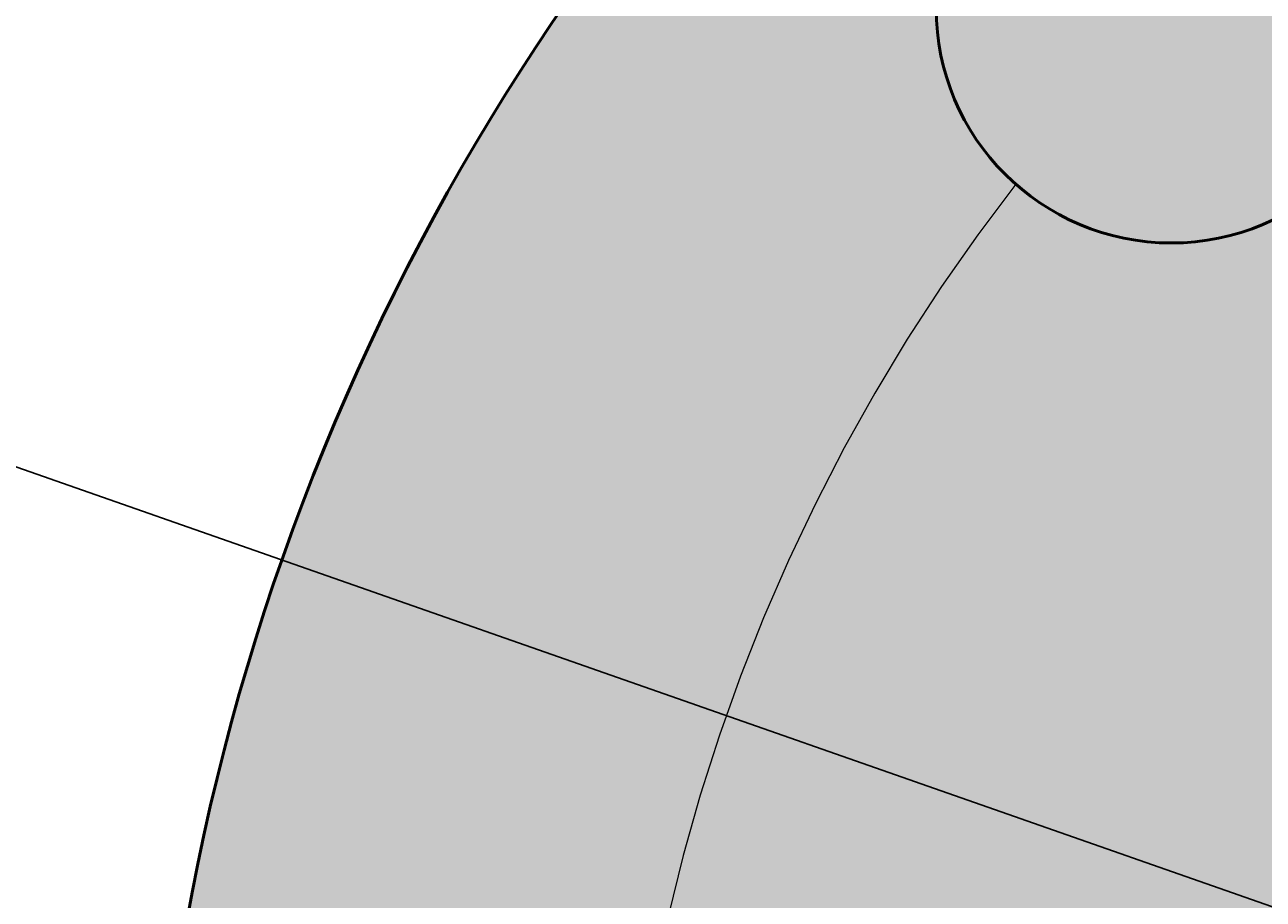
# Model space of a CAD drawing. Units: inches. Extents: x 139261 to 139415, y 52839 to 52963.
# Tile 5 of 20: x 139288 to 139314, y 52910 to 52928. Entities that reach past the tile are written whole.
import ezdxf

# ---------------------------------------------------------------- set-up
doc = ezdxf.new("R2010")
doc.units = ezdxf.units.IN
doc.header["$MEASUREMENT"] = 0
doc.linetypes.add('CENTER', pattern=[50.8, 31.75, -6.35, 6.35, -6.35])
for name, color, linetype, lineweight in [('M-CNTR', 4, 'CENTER', 18), ('M-DIMS', 2, 'Continuous', 25), ('M-HATC', 8, 'Continuous', 18), ('M-OUTL', 7, 'Continuous', 50)]:
    doc.layers.add(name, color=color, linetype=linetype, lineweight=lineweight)
doc.styles.get("Standard").update_dxf_attribs({"font": 'arial.ttf'})
doc.dimstyles.get("Standard").update_dxf_attribs({"dimtxt": 0.18, "dimasz": 0.18, "dimexe": 0.18, "dimexo": 0.0625, "dimgap": 0.09, "dimtad": 0, "dimtih": 1, "dimtoh": 1, "dimdec": 4, "dimzin": 0, "dimdsep": 46, "dimtxsty": 'Standard', "dimcen": 0.09, "dimadec": 0, "dimazin": 0, "dimtfac": 1, "dimtdec": 4, "dimtofl": 0, "dimtmove": 0, "dimatfit": 3, "dimfxl": 1, "dimtolj": 1, "dimtzin": 0, "dimarcsym": 0})

# ---------------------------------------------------------------- blocks, each defined once
blk = doc.blocks.new('*U1')
blk.add_circle((0, 0), 5)
blk = doc.blocks.new('*U2')
at = {"layer": 'M-OUTL', "color": 0, "linetype": 'ByBlock', "lineweight": -2, "transparency": 16777216, "rotation": 45.00000000000001}
blk.add_blockref('*U1', (139312.073, 52928.502), dxfattribs=at)
blk = doc.blocks.new('*D4')
at = {"layer": 'Defpoints', "color": 0, "transparency": 16777216}
for p in [(139373.053, 52923.26), (139307.661, 52877.175)]:
    blk.add_point(p, dxfattribs=at)
at = {"layer": 'M-DIMS', "color": 0, "lineweight": -2, "transparency": 16777216}
for p, q in [((139414.011, 52952.126), (139373.2, 52923.364)), ((139414.191, 52952.126), (139414.011, 52952.126)), ((139340.267, 52900.217), (139340.447, 52900.217)), ((139340.357, 52900.127), (139340.357, 52900.307))]:
    blk.add_line(p, q, dxfattribs=at)
blk.add_arc((139340.357, 52900.217), 40, 34.9168, 52.0771, dxfattribs=at)
at = {"layer": 'M-DIMS', "color": 0, "transparency": 16777216}
blk.add_solid([(139373.183, 52923.388), (139373.217, 52923.339), (139373.053, 52923.26)], dxfattribs=at)
at = {"layer": 'M-DIMS', "color": 0, "transparency": 16777216, "insert": (139414.822, 52952.126), "char_height": 0.18, "attachment_point": 5}
blk.add_mtext('\\A1;∅80.0000', dxfattribs=at)
blk = doc.blocks.new('*D5')
at = {"layer": 'Defpoints', "color": 0, "transparency": 16777216}
for p in [(139316.763, 52908.484), (139363.951, 52891.951)]:
    blk.add_point(p, dxfattribs=at)
at = {"layer": 'M-DIMS', "color": 0, "lineweight": -2, "transparency": 16777216}
for p, q in [((139262.553, 52927.414), (139262.733, 52927.414)), ((139262.733, 52927.414), (139316.593, 52908.544)), ((139340.267, 52900.217), (139340.447, 52900.217)), ((139340.357, 52900.127), (139340.357, 52900.307))]:
    blk.add_line(p, q, dxfattribs=at)
at = {"layer": 'M-DIMS', "color": 0, "transparency": 16777216}
blk.add_solid([(139316.603, 52908.572), (139316.583, 52908.515), (139316.763, 52908.484)], dxfattribs=at)
at = {"layer": 'M-DIMS', "color": 0, "transparency": 16777216, "insert": (139261.922, 52927.414), "char_height": 0.18, "attachment_point": 5}
blk.add_mtext('\\A1;∅50.0000', dxfattribs=at)
blk = doc.blocks.new('*D9')
at = {"layer": 'Defpoints', "color": 0, "transparency": 16777216}
for p in [(139302.054, 52932.357), (139378.659, 52868.078)]:
    blk.add_point(p, dxfattribs=at)
at = {"layer": 'M-DIMS', "color": 0, "lineweight": -2, "transparency": 16777216}
for p, q in [((139278.893, 52951.64), (139279.073, 52951.64)), ((139279.073, 52951.64), (139301.916, 52932.472)), ((139340.267, 52900.217), (139340.447, 52900.217)), ((139340.357, 52900.127), (139340.357, 52900.307))]:
    blk.add_line(p, q, dxfattribs=at)
at = {"layer": 'M-DIMS', "color": 0, "transparency": 16777216}
blk.add_solid([(139301.936, 52932.495), (139301.897, 52932.449), (139302.054, 52932.357)], dxfattribs=at)
at = {"layer": 'M-DIMS', "color": 0, "transparency": 16777216, "insert": (139278.506, 52951.64), "char_height": 0.18, "attachment_point": 5}
blk.add_mtext('\\A1;∅100', dxfattribs=at)

msp = doc.modelspace()

# ---------------------------------------------------------------- hatches: boundary and pattern name
at = {"layer": 'M-HATC'}
h = msp.add_hatch(color=256, dxfattribs=at)
h.dxf.hatch_style = 1
h.paths.add_polyline_path([(139290.35689, 52900.21749, 1), (139390.35689, 52900.21749, 1)])
h.paths.add_polyline_path([(139335.36666, 52939.90499, -0.01563646), (139335.35689, 52940.21749, -1), (139345.35689, 52940.21749, -0.01563646), (139345.34711, 52939.90499, -0.13461315), (139364.89157, 52931.80941, -0.691035), (139373.64116, 52928.50176, -0.21521822), (139371.94881, 52924.75216, -0.13461315), (139380.04439, 52905.20771, -0.43265224), (139385.35689, 52900.21749, -0.43265224), (139380.04439, 52895.22726, -0.13461315), (139371.94881, 52875.68281, -0.21521822), (139373.64116, 52871.93321, -0.691035), (139364.89157, 52868.62556, -0.13461315), (139345.34711, 52860.52999, -0.01563646), (139345.35689, 52860.21749, -1), (139335.35689, 52860.21749, -0.01563646), (139335.36666, 52860.52999, -0.13461315), (139315.82221, 52868.62556, -0.691035), (139307.07262, 52871.93321, -0.21521822), (139308.76496, 52875.68281, -0.13461315), (139300.66939, 52895.22726, -0.43265224), (139295.35689, 52900.21749, -0.43265224), (139300.66939, 52905.20771, -0.13461315), (139308.76496, 52924.75216, -0.21521822), (139307.07262, 52928.50176, -0.691035), (139315.82221, 52931.80941, -0.13461315)], flags=16)
h.paths.add_polyline_path([(139365.35689, 52900.21749, -1), (139315.35689, 52900.21749, -1)], flags=0)
h.paths.add_polyline_path([(139323.71474, 52911.30978), (139356.99903, 52911.30978, -0.3027197), (139356.99903, 52889.12519), (139323.71474, 52889.12519, -0.3027197)], flags=0)
h.paths.add_polyline_path([(139364.89157, 52931.80941, 0.13461315), (139345.34711, 52939.90499, -0.93933644), (139335.36666, 52939.90499, 0.13461315), (139315.82221, 52931.80941, -0.18270763), (139317.07262, 52928.50176, -0.64579494), (139308.76496, 52924.75216, 0.13461315), (139300.66939, 52905.20771, -0.39601219), (139305.35689, 52900.21749, -0.39601219), (139300.66939, 52895.22726, 0.13461315), (139308.76496, 52875.68281, -0.64579494), (139317.07262, 52871.93321, -0.18270763), (139315.82221, 52868.62556, 0.13461315), (139335.36666, 52860.52999, -0.93933644), (139345.34711, 52860.52999, 0.13461315), (139364.89157, 52868.62556, -0.18270763), (139363.64116, 52871.93321, -0.64579494), (139371.94881, 52875.68281, 0.13461315), (139380.04439, 52895.22726, -0.39601219), (139375.35689, 52900.21749, -0.39601219), (139380.04439, 52905.20771, 0.13461315), (139371.94881, 52924.75216, -0.64579494), (139363.64116, 52928.50176, -0.18270763)], flags=0)
h = msp.add_hatch(color=256, dxfattribs=at)
h.dxf.hatch_style = 1
h.set_gradient(color1=(205, 105, 40), tint=1)
h.paths.add_polyline_path([(139335.35689, 52940.21749, 1), (139345.35689, 52940.21749, 1)])
h.paths.add_polyline_path([(139307.07262, 52928.50176, 1), (139317.07262, 52928.50176, 1)])
h.paths.add_polyline_path([(139295.35689, 52900.21749, 1), (139305.35689, 52900.21749, 1)])
h.paths.add_polyline_path([(139307.07262, 52871.93321, 1), (139317.07262, 52871.93321, 1)])
h.paths.add_polyline_path([(139345.35689, 52860.21749, 1), (139335.35689, 52860.21749, 1)])
h.paths.add_polyline_path([(139363.64116, 52871.93321, 1), (139373.64116, 52871.93321, 1)])
h.paths.add_polyline_path([(139375.35689, 52900.21749, 1), (139385.35689, 52900.21749, 1)])
h.paths.add_polyline_path([(139363.64116, 52928.50176, 1), (139373.64116, 52928.50176, 1)])
h = msp.add_hatch(color=256, dxfattribs=at)
h.dxf.hatch_style = 1
h.paths.add_polyline_path([(139345.34711, 52939.90499, -0.93933644), (139335.36666, 52939.90499, 0.13461315), (139315.82221, 52931.80941, -0.18270763), (139317.07262, 52928.50176, -0.64579494), (139308.76496, 52924.75216, 0.13461315), (139300.66939, 52905.20771, -0.39601219), (139305.35689, 52900.21749, -0.39601219), (139300.66939, 52895.22726, 0.13461315), (139308.76496, 52875.68281, -0.64579494), (139317.07262, 52871.93321, -0.18270763), (139315.82221, 52868.62556, 0.13461315), (139335.36666, 52860.52999, -0.93933644), (139345.34711, 52860.52999, 0.13461315), (139364.89157, 52868.62556, -0.18270763), (139363.64116, 52871.93321, -0.64579494), (139371.94881, 52875.68281, 0.13461315), (139380.04439, 52895.22726, -0.39601219), (139375.35689, 52900.21749, -0.39601219), (139380.04439, 52905.20771, 0.13461315), (139371.94881, 52924.75216, -0.64579494), (139363.64116, 52928.50176, -0.18270763), (139364.89157, 52931.80941, 0.13461315)])
h.paths.add_polyline_path([(139365.35689, 52900.21749, -1), (139315.35689, 52900.21749, -1)], flags=16)
h.paths.add_polyline_path([(139356.99903, 52911.30978, -0.3027197), (139356.99903, 52889.12519), (139323.71474, 52889.12519, -0.3027197), (139323.71474, 52911.30978)], flags=0)

# ---------------------------------------------------------------- linework, layer by layer
at = {"layer": 'M-CNTR'}
msp.add_arc((139340.35689, 52900.21749), 40, 142.166643, 172.833357, dxfattribs=at)
at = {"layer": 'M-OUTL'}
msp.add_circle((139340.35689, 52900.21749), 50, dxfattribs=at)

# ---------------------------------------------------------------- block references
msp.add_blockref('*U2', (0, 0), dxfattribs=at)

# ---------------------------------------------------------------- dimensions: what is measured, and where the dimension line sits
at = {"layer": 'M-DIMS'}
for p1, p2, override, picture, middle in [((139307.66087, 52877.17469), (139373.0529, 52923.26028), {"dimclrd": 0, "dimclre": 0, "dimclrt": 0}, '*D4', (139414.82217, 52952.12585)), ((139378.65939, 52868.07845), (139302.05438, 52932.35652), {"dimdec": 0, "dimlfac": 1, "dimrnd": 0, "dimzin": 0, "dimdsep": 46, "dimlunit": 2}, '*D9', (139278.50641, 52951.63995)), ((139363.95063, 52891.95098), (139316.76314, 52908.48399), {"dimclrd": 0, "dimclre": 0, "dimclrt": 0}, '*D5', (139261.92224, 52927.41429))]:
    dim = msp.add_diameter_dim_2p(p1=p1, p2=p2, dimstyle='Standard', override=override, dxfattribs=at)
    dim.commit()
    dim.dimension.update_dxf_attribs({"geometry": picture, "text_midpoint": middle, "dimtype": 163})

doc.saveas('drawing.dxf')
